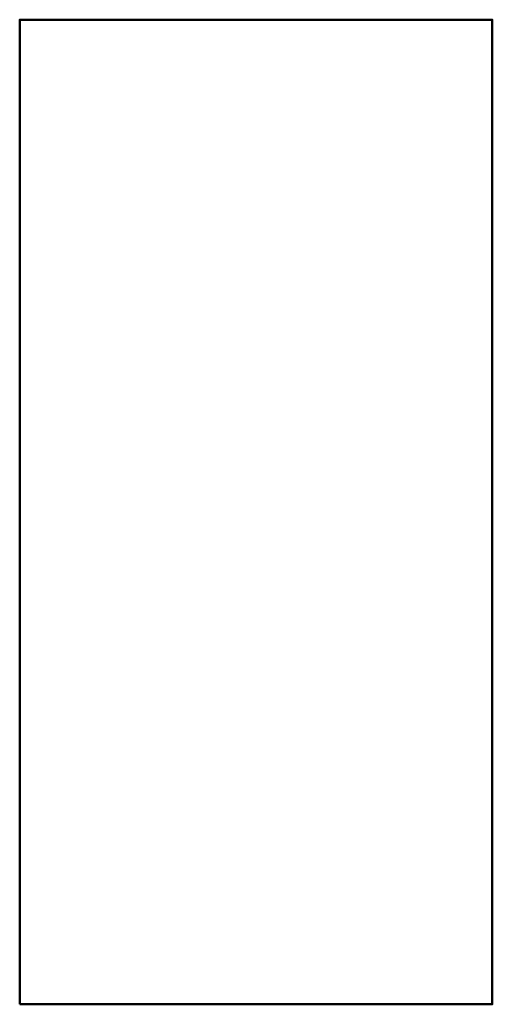
# Model space of a CAD drawing. Units: inches. Extents: x 101 to 137, y 38.6 to 113.6.
import ezdxf

# ---------------------------------------------------------------- set-up
doc = ezdxf.new("R2010")
doc.units = ezdxf.units.IN
doc.layers.add('A-ANNO-TTLB', color=7, linetype='Continuous', lineweight=50)

msp = doc.modelspace()

# ---------------------------------------------------------------- linework, layer by layer
at = {"layer": 'A-ANNO-TTLB', "elevation": 63}
msp.add_lwpolyline([(100.955, 38.628), (136.955, 38.628), (136.955, 113.628), (100.955, 113.628)], close=True, dxfattribs=at)

doc.saveas('drawing.dxf')
